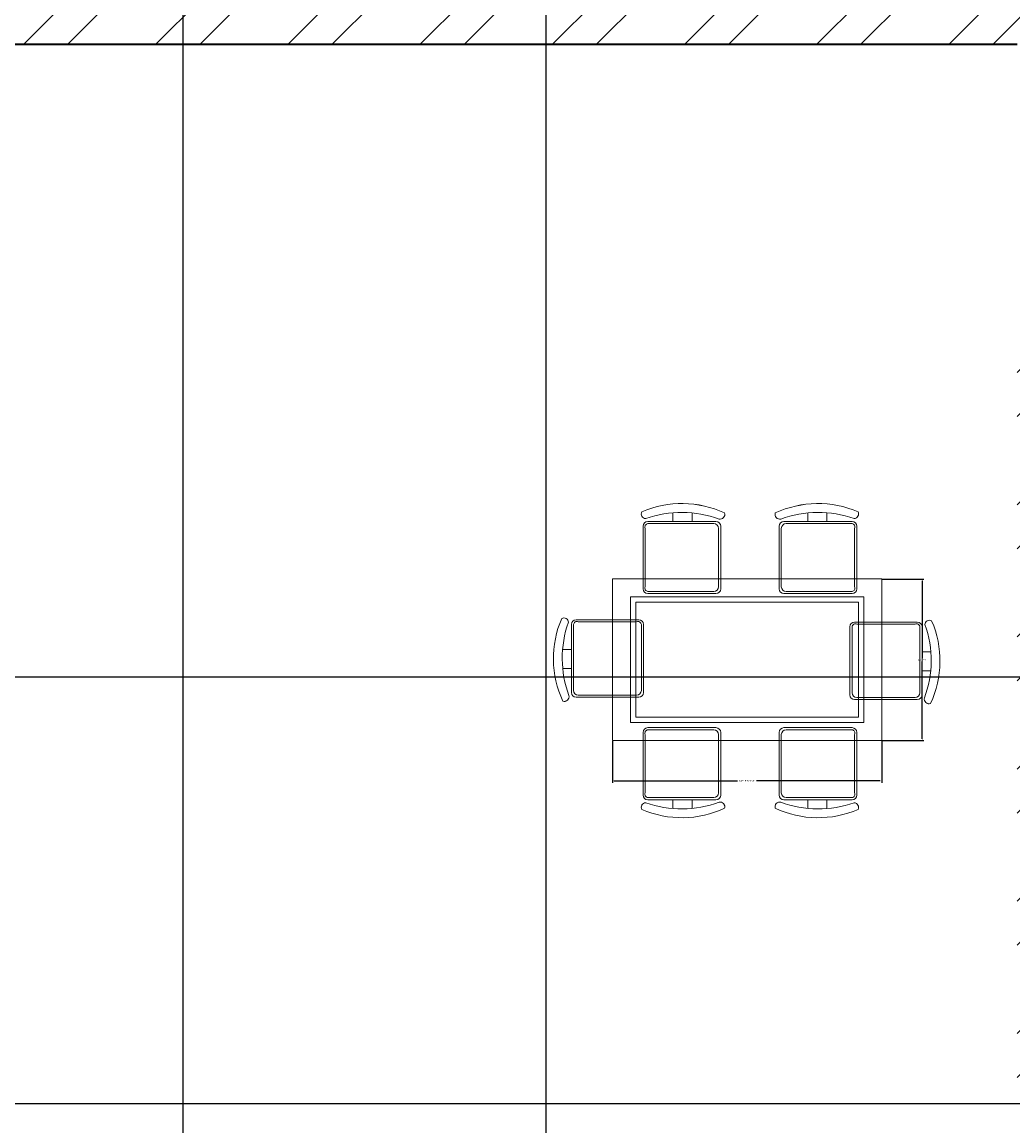
# Model space of a CAD drawing. Units: inches. Extents: x 1965 to 2673, y 1802 to 2669.
# Tile 13 of 16: x 2372 to 2473, y 2154 to 2266. Entities that reach past the tile are written whole.
import ezdxf

# ---------------------------------------------------------------- set-up
doc = ezdxf.new("R2010")
doc.units = ezdxf.units.IN
for name, color, linetype, lineweight in [('A-ANNO-DIMS', 2, 'Continuous', 18), ('A-FURN', 8, 'Continuous', 13), ('A-WALL', 7, 'Continuous', 35), ('A-WALL-PATT', 252, 'Continuous', 13)]:
    doc.layers.add(name, color=color, linetype=linetype, lineweight=lineweight)
doc.styles.get("Standard").update_dxf_attribs({"font": 'arial.ttf'})
doc.dimstyles.get("Standard").update_dxf_attribs({"dimtxt": 0.18, "dimasz": 0.18, "dimexe": 0.18, "dimexo": 0.0625, "dimgap": 0.09, "dimtad": 0, "dimtih": 1, "dimtoh": 1, "dimdec": 4, "dimzin": 0, "dimdsep": 46, "dimtxsty": 'Standard', "dimcen": 0.09, "dimadec": 0, "dimazin": 0, "dimtfac": 1, "dimtdec": 4, "dimtofl": 0, "dimtmove": 0, "dimatfit": 3, "dimfxl": 1, "dimtolj": 1, "dimtzin": 0, "dimarcsym": 0})

# ---------------------------------------------------------------- blocks, each defined once
blk = doc.blocks.new('TABLE-DINING-RECT')
for points in [[(0, 16.47), (27.44, 16.47), (27.44, 0), (0, 0)], [(0, 16.47), (27.44, 16.47), (27.44, 0), (0, 0)], [(1.83, 14.64), (25.61, 14.64), (25.61, 1.83), (1.83, 1.83)], [(1.83, 14.64), (25.61, 14.64), (25.61, 1.83), (1.83, 1.83)], [(2.38, 14.09), (25.06, 14.09), (25.06, 2.38), (2.38, 2.38)], [(2.38, 14.09), (25.06, 14.09), (25.06, 2.38), (2.38, 2.38)]]:
    blk.add_lwpolyline(points, close=True)
blk = doc.blocks.new('*D19')
at = {"layer": 'A-ANNO-DIMS', "color": 0, "lineweight": -2, "transparency": 16777216}
for p, q in [((2431.84, 2193.05), (2431.84, 2188.82)), ((2459.28, 2193.05), (2459.28, 2188.82)), ((2432.02, 2189), (2444.6, 2189)), ((2459.1, 2189), (2446.52, 2189))]:
    blk.add_line(p, q, dxfattribs=at)
at = {"layer": 'A-ANNO-DIMS', "color": 0, "transparency": 16777216}
for points in [[(2432.02, 2189.03), (2432.02, 2188.97), (2431.84, 2189)], [(2459.1, 2189.03), (2459.1, 2188.97), (2459.28, 2189)]]:
    blk.add_solid(points, dxfattribs=at)
at = {"layer": 'Defpoints', "color": 0, "transparency": 16777216}
for p in [(2431.84, 2193.12), (2459.28, 2193.12), (2459.28, 2189)]:
    blk.add_point(p, dxfattribs=at)
at = {"layer": 'A-ANNO-DIMS', "color": 0, "transparency": 16777216, "insert": (2445.56, 2189), "char_height": 0.18, "attachment_point": 5}
blk.add_mtext('\\A1;TABLE 27 TYP.', dxfattribs=at)
blk = doc.blocks.new('*D20')
at = {"layer": 'A-ANNO-DIMS', "color": 0, "lineweight": -2, "transparency": 16777216}
for p, q in [((2459.34, 2209.58), (2463.58, 2209.58)), ((2463.4, 2209.4), (2463.4, 2201.53)), ((2463.4, 2193.3), (2463.4, 2201.17)), ((2459.34, 2193.12), (2463.58, 2193.12))]:
    blk.add_line(p, q, dxfattribs=at)
at = {"layer": 'A-ANNO-DIMS', "color": 0, "transparency": 16777216}
for points in [[(2463.37, 2209.4), (2463.43, 2209.4), (2463.4, 2209.58)], [(2463.37, 2193.3), (2463.43, 2193.3), (2463.4, 2193.12)]]:
    blk.add_solid(points, dxfattribs=at)
at = {"layer": 'Defpoints', "color": 0, "transparency": 16777216}
for p in [(2459.28, 2209.58), (2463.4, 2209.58), (2459.28, 2193.12)]:
    blk.add_point(p, dxfattribs=at)
at = {"layer": 'A-ANNO-DIMS', "color": 0, "transparency": 16777216, "insert": (2463.4, 2201.35), "char_height": 0.18, "attachment_point": 5}
blk.add_mtext('\\A1;16 TYP.', dxfattribs=at)
blk = doc.blocks.new('*D47')
at = {"layer": 'A-ANNO-DIMS', "color": 0, "lineweight": -2, "transparency": 16777216}
for p, q in [((2573.53, 2199.58), (2012.19, 2199.58)), ((2012.37, 2199.4), (2012.37, 2178.02)), ((2012.37, 2156.27), (2012.37, 2177.65)), ((2573.53, 2156.09), (2012.19, 2156.09))]:
    blk.add_line(p, q, dxfattribs=at)
at = {"layer": 'A-ANNO-DIMS', "color": 0, "transparency": 16777216}
for points in [[(2012.34, 2199.4), (2012.4, 2199.4), (2012.37, 2199.58)], [(2012.34, 2156.27), (2012.4, 2156.27), (2012.37, 2156.09)]]:
    blk.add_solid(points, dxfattribs=at)
at = {"layer": 'Defpoints', "color": 0, "transparency": 16777216}
for p in [(2012.37, 2199.58), (2573.59, 2199.58), (2573.59, 2156.09)]:
    blk.add_point(p, dxfattribs=at)
at = {"layer": 'A-ANNO-DIMS', "color": 0, "transparency": 16777216, "insert": (2012.37, 2177.83), "char_height": 0.18, "attachment_point": 5}
blk.add_mtext('\\A1;43.48', dxfattribs=at)
blk = doc.blocks.new('*D50')
at = {"layer": 'A-ANNO-DIMS', "color": 0, "lineweight": -2, "transparency": 16777216}
for p, q in [((2388.09, 2116.15), (2388.09, 2600.5)), ((2388.27, 2600.32), (2406.37, 2600.32)), ((2424.91, 2600.32), (2406.81, 2600.32)), ((2425.09, 2116.15), (2425.09, 2600.5))]:
    blk.add_line(p, q, dxfattribs=at)
at = {"layer": 'A-ANNO-DIMS', "color": 0, "transparency": 16777216}
for points in [[(2388.27, 2600.35), (2388.27, 2600.29), (2388.09, 2600.32)], [(2424.91, 2600.35), (2424.91, 2600.29), (2425.09, 2600.32)]]:
    blk.add_solid(points, dxfattribs=at)
at = {"layer": 'Defpoints', "color": 0, "transparency": 16777216}
for p in [(2425.09, 2600.32), (2388.09, 2116.09), (2425.09, 2116.09)]:
    blk.add_point(p, dxfattribs=at)
at = {"layer": 'A-ANNO-DIMS', "color": 0, "transparency": 16777216, "insert": (2406.59, 2600.32), "char_height": 0.18, "attachment_point": 5}
blk.add_mtext('\\A1;37', dxfattribs=at)

msp = doc.modelspace()

# ---------------------------------------------------------------- hatches: boundary and pattern name
at = {"layer": 'A-WALL-PATT'}
h = msp.add_hatch(dxfattribs=at)
h.set_pattern_fill('ANSI32', color=256)
h.paths.add_polyline_path([(2051.5927, 2561.0914), (2076.7559, 2561.0914), (2076.7559, 2563.3414), (2076.7559, 2565.5914), (2047.0927, 2565.5914), (2047.0927, 2518.3824), (2051.5927, 2518.3824)])
h.paths.add_polyline_path([(2051.5927, 2458.3824), (2049.3427, 2458.3824), (2047.0927, 2458.3824), (2047.0927, 2412.5914), (2248.0927, 2412.5914), (2248.0927, 2268.5914), (2252.5927, 2268.5914), (2252.5927, 2412.5914), (2252.5927, 2421.0404), (2250.3427, 2421.0404), (2248.0927, 2421.0404), (2248.0927, 2417.0914), (2051.5927, 2417.0914)])
h.paths.add_polyline_path([(2211.4933, 2268.5914), (2104.0927, 2268.5914), (2104.0927, 2272.4654), (2101.8427, 2272.4654), (2099.5927, 2272.4654), (2099.5927, 2268.5914), (2051.5927, 2268.5914), (2051.5927, 2264.0914), (2147.5927, 2264.0914), (2147.5927, 2259.8893), (2152.0927, 2259.8893), (2152.0927, 2264.0914), (2211.4933, 2264.0914), (2211.4933, 2266.3414)])
h.paths.add_polyline_path([(2104.0927, 2376.0914), (2099.5927, 2376.0914), (2047.0927, 2376.0914), (2047.0927, 2333.0682), (2051.5927, 2333.0682), (2051.5927, 2371.5914), (2099.5927, 2371.5914), (2099.5927, 2293.6123), (2104.0927, 2293.6123)], flags=17)
h.paths.add_polyline_path([(2051.5927, 2309.0682), (2047.0927, 2309.0682), (2047.0927, 2233.5821), (2051.5927, 2233.5821)])
h.paths.add_polyline_path([(2104.0927, 2412.5914), (2099.5927, 2412.5914), (2099.5927, 2376.0914), (2104.0927, 2376.0914)], flags=17)
h.paths.add_polyline_path([(2290.1254, 2268.5914), (2242.4924, 2268.5914), (2242.4924, 2264.0914), (2290.1254, 2264.0914), (2290.1254, 2266.3414)])
h.paths.add_polyline_path([(2284.653, 2264.0914), (2280.153, 2264.0914), (2280.153, 2161.6826), (2284.653, 2161.6826)])
h.paths.add_polyline_path([(2578.0927, 2329.4656), (2573.5927, 2329.4656), (2573.5927, 2268.5914), (2525.5927, 2268.5914), (2525.5927, 2271.9222), (2523.3427, 2271.9222), (2521.0927, 2271.9222), (2521.0927, 2268.5914), (2324.2835, 2268.5914), (2324.2835, 2264.0914), (2329.0927, 2264.0914), (2329.0927, 2259.4977), (2333.5927, 2259.4977), (2333.5927, 2264.0914), (2473.0927, 2264.0914), (2473.0927, 2259.9371), (2477.5927, 2259.9371), (2477.5927, 2264.0914), (2573.5927, 2264.0914), (2573.5927, 2235.5751), (2578.0927, 2235.5751)])
h.paths.add_polyline_path([(2377.0927, 2412.5914), (2578.0927, 2412.5914), (2578.0927, 2444.2286), (2575.8427, 2444.2286), (2573.5927, 2444.2286), (2573.5927, 2417.0914), (2429.5927, 2417.0914), (2377.0927, 2417.0914), (2377.0927, 2421.7443), (2372.5927, 2421.7443), (2372.5927, 2268.5914), (2377.0927, 2268.5914)])
h.paths.add_polyline_path([(2525.5927, 2371.5914), (2573.5927, 2371.5914), (2573.5927, 2353.4656), (2578.0927, 2353.4656), (2578.0927, 2376.0914), (2525.5927, 2376.0914), (2521.0927, 2376.0914), (2521.0927, 2290.6472), (2525.5927, 2290.6472)], flags=17)
h.paths.add_polyline_path([(2477.5927, 2236.4106), (2475.3427, 2236.4106), (2473.0927, 2236.4106), (2473.0927, 2084.5914), (2465.3309, 2084.5914), (2465.3309, 2080.0914), (2481.6764, 2080.0914), (2481.6764, 2082.3414), (2481.6764, 2084.5914), (2477.5927, 2084.5914), (2477.5927, 2151.5914), (2573.5927, 2151.5914), (2573.5927, 2130.2907), (2578.0927, 2130.2907), (2578.0927, 2199.5751), (2575.8427, 2199.5751), (2573.5927, 2199.5751), (2573.5927, 2156.0914), (2477.5927, 2156.0914)])
h.paths.add_polyline_path([(2573.5927, 2084.5914), (2505.5513, 2084.5914), (2505.5513, 2080.0914), (2573.5927, 2080.0914)], flags=17)
h.paths.add_polyline_path([(2578.0927, 2106.2907), (2575.8427, 2106.2907), (2573.5927, 2106.2907), (2573.5927, 2050.8986), (2578.0927, 2050.8986)])
h.paths.add_polyline_path([(2578.0927, 1990.8986), (2575.8427, 1990.8986), (2573.5927, 1990.8986), (2573.5927, 1936.0914), (2522.132, 1936.0914), (2522.132, 1931.5914), (2578.0927, 1931.5914)])
h.paths.add_polyline_path([(2462.132, 1936.0914), (2429.5927, 1936.0914), (2429.5927, 2080.0914), (2432.623, 2080.0914), (2432.623, 2082.3414), (2432.623, 2084.5914), (2429.5927, 2084.5914), (2429.5927, 2120.5914), (2333.5927, 2120.5914), (2333.5927, 2229.3125), (2331.3427, 2229.3125), (2329.0927, 2229.3125), (2329.0927, 2116.0914), (2425.0927, 2116.0914), (2425.0927, 1936.0914), (2346.4058, 1936.0914), (2346.4058, 1931.5914), (2462.132, 1931.5914), (2462.132, 1933.8414)])
h.paths.add_polyline_path([(2211.767, 1933.8414), (2211.767, 1936.0914), (2200.0927, 1936.0914), (2200.0927, 2080.0914), (2200.0927, 2116.0914), (2284.653, 2116.0914), (2284.653, 2130.591), (2282.403, 2130.591), (2280.153, 2130.591), (2280.153, 2120.5914), (2200.0927, 2120.5914), (2195.5927, 2120.5914), (2195.5927, 2080.0914), (2195.5927, 1936.0914), (2139.0533, 1936.0914), (2139.0533, 1931.5914), (2211.767, 1931.5914)])
h.paths.add_polyline_path([(2282.2502, 1933.8414), (2282.2502, 1936.0914), (2259.767, 1936.0914), (2259.767, 1931.5914), (2282.2502, 1931.5914)], flags=17)
h.paths.add_polyline_path([(2051.5927, 1987.096), (2049.3427, 1987.096), (2047.0927, 1987.096), (2047.0927, 1931.5914), (2079.0533, 1931.5914), (2079.0533, 1933.8414), (2079.0533, 1936.0914), (2051.5927, 1936.0914)])
h.paths.add_polyline_path([(2051.5927, 2197.5821), (2049.3427, 2197.5821), (2047.0927, 2197.5821), (2047.0927, 2141.952), (2051.5927, 2141.952), (2051.5927, 2151.5914), (2147.5927, 2151.5914), (2147.5927, 2084.5914), (2144.3652, 2084.5914), (2144.3652, 2080.0914), (2155.9662, 2080.0914), (2155.9662, 2082.3414), (2155.9662, 2084.5914), (2152.0927, 2084.5914), (2152.0927, 2239.4921), (2149.8427, 2239.4921), (2147.5927, 2239.4921), (2147.5927, 2156.0914), (2051.5927, 2156.0914)])
h.paths.add_polyline_path([(2051.5927, 2080.0914), (2123.8575, 2080.0914), (2123.8575, 2082.3414), (2123.8575, 2084.5914), (2051.5927, 2084.5914), (2051.5927, 2117.952), (2047.0927, 2117.952), (2047.0927, 2047.096), (2051.5927, 2047.096)])

# ---------------------------------------------------------------- linework, layer by layer
at = {"layer": 'A-FURN'}
for points in [[(2435.2306, 2215.7448, -0.17580919), (2442.706, 2215.6881, 0.57839206), (2443.2723, 2216.3109, 0.21452438), (2434.8341, 2216.4241, 0.55201397), (2435.2306, 2215.7447, -0.06507904)], [(2435.2306, 2215.7445, -0.17580919), (2442.706, 2215.6879, 0.57839206), (2443.2723, 2216.3106, 0.21452438), (2434.8342, 2216.4238, 0.55201397), (2435.2306, 2215.7445, -0.06507904)], [(2439.9512, 2215.4447), (2439.9512, 2216.3224, -0.06475861)], [(2439.9512, 2215.4444), (2439.9512, 2216.3221, -0.06475861)], [(2448.9994, 2215.6881, -0.57839206), (2448.433, 2216.3109, -0.21452438), (2456.8712, 2216.4241, -0.55201397), (2456.4748, 2215.7447, 0.1758092), (2448.9994, 2215.6881)], [(2448.9994, 2215.6879, -0.57839206), (2448.4331, 2216.3106, -0.21452438), (2456.8712, 2216.4238, -0.55201397), (2456.4748, 2215.7445, 0.1758092), (2448.9994, 2215.6879)], [(2451.7542, 2215.4447), (2451.7542, 2216.3224, 0.06475861)], [(2451.7542, 2215.4444), (2451.7542, 2216.3221, 0.06475861)], [(2442.3889, 2215.4447), (2435.4489, 2215.4447, 0.41421356), (2434.9634, 2214.9592), (2434.9634, 2208.578, 0.41421356), (2435.4489, 2208.0925), (2442.3889, 2208.0925, 0.41421356), (2442.8744, 2208.578), (2442.8744, 2214.9592, 0.41421356), (2442.3889, 2215.4447)], [(2442.3889, 2215.4444), (2435.4489, 2215.4444, 0.41421356), (2434.9634, 2214.9589), (2434.9634, 2208.5778, 0.41421356), (2435.4489, 2208.0922), (2442.3889, 2208.0922, 0.41421356), (2442.8744, 2208.5778), (2442.8744, 2214.9589, 0.41421356), (2442.3889, 2215.4444)], [(2456.2565, 2215.4447, -0.41421356), (2456.742, 2214.9592), (2456.742, 2208.578, -0.41421356), (2456.2565, 2208.0925), (2449.3165, 2208.0925, -0.41421356), (2448.831, 2208.578), (2448.831, 2214.9592, -0.41421356), (2449.3165, 2215.4447), (2456.2565, 2215.4447)], [(2456.2565, 2215.4444, -0.41421356), (2456.742, 2214.9589), (2456.742, 2208.5778, -0.41421356), (2456.2565, 2208.0922), (2449.3165, 2208.0922, -0.41421356), (2448.831, 2208.5778), (2448.831, 2214.9589, -0.41421356), (2449.3165, 2215.4444), (2456.2565, 2215.4444)], [(2427.4098, 2197.6927, -0.57839206), (2426.7871, 2197.1264, -0.21452438), (2426.6739, 2205.5646, -0.55201397), (2427.3532, 2205.1681, 0.17580937), (2427.4098, 2197.6927)], [(2427.4098, 2197.6924, -0.57839206), (2426.7871, 2197.1261, -0.21452438), (2426.6739, 2205.5643, -0.55201397), (2427.3532, 2205.1679, 0.17580937), (2427.4098, 2197.6924)], [(2427.6532, 2204.9498, -0.41421356), (2428.1388, 2205.4353), (2434.5199, 2205.4353, -0.41421356), (2435.0054, 2204.9498), (2435.0054, 2198.0099, -0.41421356), (2434.5199, 2197.5243), (2428.1388, 2197.5243, -0.41421356), (2427.6532, 2198.0099), (2427.6532, 2204.9498)], [(2427.6533, 2204.9495, -0.41421356), (2428.1388, 2205.435), (2434.5199, 2205.435, -0.41421356), (2435.0055, 2204.9495), (2435.0055, 2198.0096, -0.41421356), (2434.5199, 2197.524), (2428.1388, 2197.524, -0.41421356), (2427.6533, 2198.0096), (2427.6533, 2204.9495)], [(2463.3907, 2204.7121, 0.41421356), (2462.9052, 2205.1976), (2456.524, 2205.1976, 0.41421356), (2456.0385, 2204.7121), (2456.0385, 2197.7722, 0.41421356), (2456.524, 2197.2866), (2462.9052, 2197.2866, 0.41421356), (2463.3907, 2197.7722), (2463.3907, 2204.7121)], [(2463.3907, 2204.7118, 0.41421356), (2462.9052, 2205.1974), (2456.5241, 2205.1974, 0.41421356), (2456.0385, 2204.7118), (2456.0385, 2197.7719, 0.41421356), (2456.5241, 2197.2864), (2462.9052, 2197.2864, 0.41421356), (2463.3907, 2197.7719), (2463.3907, 2204.7118)], [(2463.6907, 2204.9305, -0.17580919), (2463.6341, 2197.455, 0.57839206), (2464.2568, 2196.8887, 0.21452438), (2464.3701, 2205.3269, 0.55201397), (2463.6907, 2204.9305, -0.06507904)], [(2463.6908, 2204.9302, -0.17580919), (2463.6341, 2197.4547, 0.57839206), (2464.2569, 2196.8884, 0.21452438), (2464.3701, 2205.3266, 0.55201397), (2463.6908, 2204.9302, -0.06507904)], [(2427.6532, 2200.4475), (2426.7756, 2200.4475, 0.06475861)], [(2427.6533, 2200.4472), (2426.7756, 2200.4472, 0.06475861)], [(2463.3907, 2200.2098), (2464.2684, 2200.2098, -0.06475861)], [(2463.3907, 2200.2095), (2464.2684, 2200.2095, -0.06475861)], [(2442.3889, 2187.079), (2435.4489, 2187.079, -0.41421356), (2434.9634, 2187.5645), (2434.9634, 2193.9456, -0.41421356), (2435.4489, 2194.4312), (2442.3889, 2194.4312, -0.41421356), (2442.8744, 2193.9456), (2442.8744, 2187.5645, -0.41421356), (2442.3889, 2187.079)], [(2442.3889, 2187.0787), (2435.4489, 2187.0787, -0.41421356), (2434.9634, 2187.5642), (2434.9634, 2193.9454, -0.41421356), (2435.4489, 2194.4309), (2442.3889, 2194.4309, -0.41421356), (2442.8744, 2193.9454), (2442.8744, 2187.5642, -0.41421356), (2442.3889, 2187.0787)], [(2456.2565, 2187.079, 0.41421356), (2456.742, 2187.5645), (2456.742, 2193.9456, 0.41421356), (2456.2565, 2194.4312), (2449.3165, 2194.4312, 0.41421356), (2448.831, 2193.9456), (2448.831, 2187.5645, 0.41421356), (2449.3165, 2187.079), (2456.2565, 2187.079)], [(2456.2565, 2187.0787, 0.41421356), (2456.742, 2187.5642), (2456.742, 2193.9454, 0.41421356), (2456.2565, 2194.4309), (2449.3165, 2194.4309, 0.41421356), (2448.831, 2193.9454), (2448.831, 2187.5642, 0.41421356), (2449.3165, 2187.0787), (2456.2565, 2187.0787)], [(2439.9512, 2187.079), (2439.9512, 2186.2013, 0.06475861)], [(2439.9512, 2187.0787), (2439.9512, 2186.201, 0.06475861)], [(2451.7542, 2187.079), (2451.7542, 2186.2013, -0.06475861)], [(2451.7542, 2187.0787), (2451.7542, 2186.201, -0.06475861)], [(2442.706, 2186.8356, -0.57839206), (2443.2723, 2186.2128, -0.21452438), (2434.8341, 2186.0996, -0.55201397), (2435.2306, 2186.7789, 0.17580929), (2442.706, 2186.8356)], [(2442.706, 2186.8353, -0.57839206), (2443.2723, 2186.2126, -0.21452438), (2434.8342, 2186.0993, -0.55201397), (2435.2306, 2186.7787, 0.17580929), (2442.706, 2186.8353)], [(2456.4748, 2186.7789, -0.17580928), (2448.9994, 2186.8356, 0.57839206), (2448.433, 2186.2128, 0.21452438), (2456.8712, 2186.0996, 0.55201397), (2456.4748, 2186.7789, -0.06507904)], [(2456.4748, 2186.7787, -0.17580928), (2448.9994, 2186.8353, 0.57839206), (2448.4331, 2186.2126, 0.21452438), (2456.8712, 2186.0993, 0.55201397), (2456.4748, 2186.7787, -0.06507904)]]:
    msp.add_lwpolyline(points, format="xyb", dxfattribs=at)
for points in [[(2438.0086, 2216.3384), (2438.0086, 2215.4447)], [(2438.0086, 2216.3381), (2438.0086, 2215.4444)], [(2453.6968, 2216.3384), (2453.6968, 2215.4447)], [(2453.6968, 2216.3381), (2453.6968, 2215.4444)], [(2426.7596, 2202.3901), (2427.6532, 2202.3901)], [(2426.7596, 2202.3898), (2427.6533, 2202.3898)], [(2464.2843, 2202.1524), (2463.3907, 2202.1524)], [(2464.2844, 2202.1521), (2463.3907, 2202.1521)], [(2438.0086, 2186.1853), (2438.0086, 2187.079)], [(2438.0086, 2186.185), (2438.0086, 2187.0787)], [(2453.6968, 2186.1853), (2453.6968, 2187.079)], [(2453.6968, 2186.185), (2453.6968, 2187.0787)]]:
    msp.add_lwpolyline(points, dxfattribs=at)
for points in [[(2435.4519, 2215.226), (2442.1701, 2215.226, -0.41421356), (2442.6556, 2214.7405), (2442.6556, 2208.7968, -0.41421356), (2442.1701, 2208.3113), (2435.4519, 2208.3113, -0.51206948), (2435.1821, 2208.7968), (2435.1821, 2214.7405, -0.51206948)], [(2435.4519, 2215.2257), (2442.1701, 2215.2257, -0.41421356), (2442.6557, 2214.7402), (2442.6557, 2208.7965, -0.41421356), (2442.1701, 2208.311), (2435.4519, 2208.311, -0.51206948), (2435.1821, 2208.7965), (2435.1821, 2214.7402, -0.51206948)], [(2456.2535, 2215.226), (2449.5352, 2215.226, 0.41421356), (2449.0497, 2214.7405), (2449.0497, 2208.7968, 0.41421356), (2449.5352, 2208.3113), (2456.2535, 2208.3113, 0.51206948), (2456.5232, 2208.7968), (2456.5232, 2214.7405, 0.51206948)], [(2456.2535, 2215.2257), (2449.5353, 2215.2257, 0.41421356), (2449.0497, 2214.7402), (2449.0497, 2208.7965, 0.41421356), (2449.5353, 2208.311), (2456.2535, 2208.311, 0.51206948), (2456.5233, 2208.7965), (2456.5233, 2214.7402, 0.51206948)], [(2427.872, 2204.9469), (2427.872, 2198.2286, 0.41421356), (2428.3575, 2197.7431), (2434.3012, 2197.7431, 0.41421356), (2434.7867, 2198.2286), (2434.7867, 2204.9469, 0.51206948), (2434.3012, 2205.2166), (2428.3575, 2205.2166, 0.51206948)], [(2427.872, 2204.9466), (2427.872, 2198.2283, 0.41421356), (2428.3575, 2197.7428), (2434.3012, 2197.7428, 0.41421356), (2434.7867, 2198.2283), (2434.7867, 2204.9466, 0.51206948), (2434.3012, 2205.2163), (2428.3575, 2205.2163, 0.51206948)], [(2463.172, 2204.7092), (2463.172, 2197.9909, -0.41421356), (2462.6865, 2197.5054), (2456.7428, 2197.5054, -0.41421356), (2456.2572, 2197.9909), (2456.2572, 2204.7092, -0.51206948), (2456.7428, 2204.9789), (2462.6865, 2204.9789, -0.51206948)], [(2463.172, 2204.7089), (2463.172, 2197.9906, -0.41421356), (2462.6865, 2197.5051), (2456.7428, 2197.5051, -0.41421356), (2456.2573, 2197.9906), (2456.2573, 2204.7089, -0.51206948), (2456.7428, 2204.9786), (2462.6865, 2204.9786, -0.51206948)], [(2435.4519, 2187.2977), (2442.1701, 2187.2977, 0.41421356), (2442.6556, 2187.7832), (2442.6556, 2193.7269, 0.41421356), (2442.1701, 2194.2124), (2435.4519, 2194.2124, 0.51206948), (2435.1821, 2193.7269), (2435.1821, 2187.7832, 0.51206948)], [(2435.4519, 2187.2974), (2442.1701, 2187.2974, 0.41421356), (2442.6557, 2187.7829), (2442.6557, 2193.7266, 0.41421356), (2442.1701, 2194.2121), (2435.4519, 2194.2121, 0.51206948), (2435.1821, 2193.7266), (2435.1821, 2187.7829, 0.51206948)], [(2456.2535, 2187.2977), (2449.5352, 2187.2977, -0.41421356), (2449.0497, 2187.7832), (2449.0497, 2193.7269, -0.41421356), (2449.5352, 2194.2124), (2456.2535, 2194.2124, -0.51206948), (2456.5232, 2193.7269), (2456.5232, 2187.7832, -0.51206948)], [(2456.2535, 2187.2974), (2449.5353, 2187.2974, -0.41421356), (2449.0497, 2187.7829), (2449.0497, 2193.7266, -0.41421356), (2449.5353, 2194.2121), (2456.2535, 2194.2121, -0.51206948), (2456.5233, 2193.7266), (2456.5233, 2187.7829, -0.51206948)]]:
    msp.add_lwpolyline(points, format="xyb", close=True, dxfattribs=at)
at = {"layer": 'A-WALL'}
msp.add_line((2333.5927, 2264.0914), (2473.0927, 2264.0914), dxfattribs=at)

# ---------------------------------------------------------------- block references
at = {"layer": 'A-FURN'}
msp.add_blockref('TABLE-DINING-RECT', (2431.8388, 2193.1139), dxfattribs=at)

# ---------------------------------------------------------------- dimensions: what is measured, and where the dimension line sits
at = {"layer": 'A-ANNO-DIMS'}
dim = msp.add_linear_dim(base=(2425.0927, 2600.3164), p1=(2388.0925, 2116.0914), p2=(2425.0927, 2116.0914), dimstyle='Standard', override={"dimdec": 0, "dimlfac": 1, "dimrnd": 0, "dimzin": 0, "dimdsep": 46, "dimlunit": 2}, dxfattribs=at)
dim.commit()
dim.dimension.update_dxf_attribs({"geometry": '*D50', "text_midpoint": (2406.5926, 2600.3164)})
dim = msp.add_linear_dim(base=(2463.3984, 2209.5838), p1=(2459.2816, 2193.116), p2=(2459.2816, 2209.5838), angle=90, text='<> TYP.', dimstyle='Standard', override={"dimdec": 0, "dimlfac": 1, "dimrnd": 0, "dimzin": 0, "dimdsep": 46, "dimlunit": 2}, dxfattribs=at)
dim.commit()
dim.dimension.update_dxf_attribs({"geometry": '*D20', "text_midpoint": (2463.3984, 2201.3499)})
dim = msp.add_linear_dim(base=(2012.3677, 2199.5751), p1=(2573.5927, 2156.0914), p2=(2573.5927, 2199.5751), angle=90, dimstyle='Standard', override={"dimdec": 2, "dimlfac": 1, "dimrnd": 0, "dimzin": 0, "dimdsep": 46, "dimlunit": 2}, dxfattribs=at)
dim.commit()
dim.dimension.update_dxf_attribs({"geometry": '*D47', "text_midpoint": (2012.3677, 2177.8332)})
dim = msp.add_linear_dim(base=(2459.2816, 2188.9992), p1=(2431.8358, 2193.116), p2=(2459.2816, 2193.116), text='TABLE <> TYP.', dimstyle='Standard', override={"dimdec": 0, "dimlfac": 1, "dimrnd": 0, "dimzin": 0, "dimdsep": 46, "dimlunit": 2}, dxfattribs=at)
dim.commit()
dim.dimension.update_dxf_attribs({"geometry": '*D19', "text_midpoint": (2445.5587, 2188.9992)})

doc.saveas('drawing.dxf')
